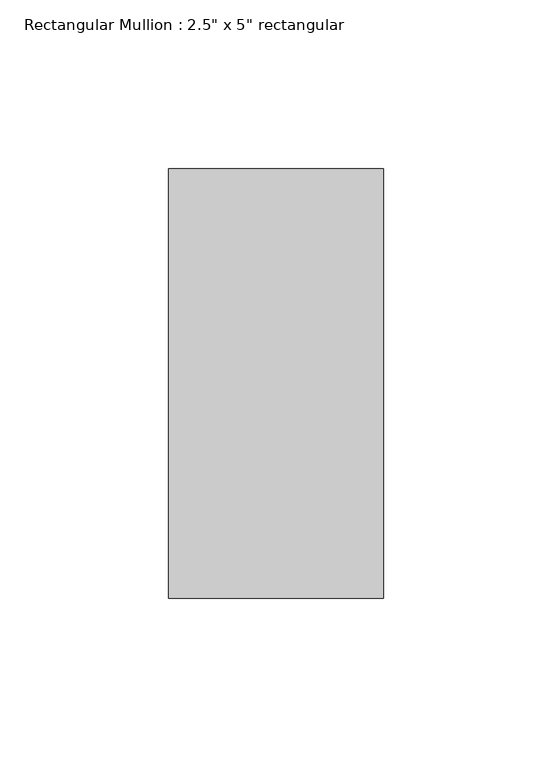
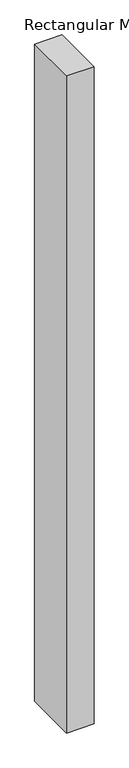
"""IFC4 building model written with IfcOpenShell, lengths in millimetres: member geometry."""

from ifc_helpers import new_model, si_unit, frame, origin, place, context, project, spatial, polyline, outline, extrude, source, transform, mapped, element, save


def member_520fb4b3(model_context):
    return source(origin(), model_context, "Body", "SweptSolid", [
        extrude(outline(polyline([(0.0, 63.5), (0.0, -63.5), (-63.5, -63.5), (-63.5, 63.5), (0.0, 63.5)])), frame((0.0, 0.0, -1601.4580508), z_axis=(0.0, 0.0, 1.0), x_axis=(1.0, 0.0, 0.0)), (0.0, 0.0, 1.0), 1601.4580508),
    ])


if __name__ == "__main__":
    model = new_model("IFC4")
    model_context = context("Model", 3, world=origin())
    ifc_project = project(units=[si_unit("LENGTHUNIT", "METRE", prefix="MILLI")], contexts=[model_context])
    site = spatial("IfcSite", under=ifc_project)
    building = spatial("IfcBuilding", under=site)
    placement = place(None, origin())
    member_shape = member_520fb4b3(model_context)
    element("IfcMember", 1, ObjectType="Rectangular Mullion : 2.5\" x 5\" rectangular", at=placement, inside=building, context=model_context, shape_type="MappedRepresentation", body=[
        mapped(member_shape, transform((0.0, 0.0, 0.0), x_axis=(1.0, 0.0, 0.0), y_axis=(0.0, 1.0, 0.0), z_axis=(0.0, 0.0, 1.0))),
    ])
    save(model, "model.ifc")

# Revit data of these elements
# Type "Rectangular Mullion : 2.5\" x 5\" rectangular"
#   built-in parameter 1007304 = 0.416667 (stored number, unit not read)
#   built-in parameter 1007301 = 0.104167 (stored number, unit not read)
#   built-in parameter 1007300 = 0.104167 (stored number, unit not read)
# Element 1 (IfcMember, "Rectangular Mullion : 2.5\" x 5\" rectangular")
#   Materials on its faces: "Aluminum"
# Materials
#   "Aluminum": class "Metal", colour RGB 247 247 247, transparency 0, Description = "Aluminum 6061", Cost = 0
